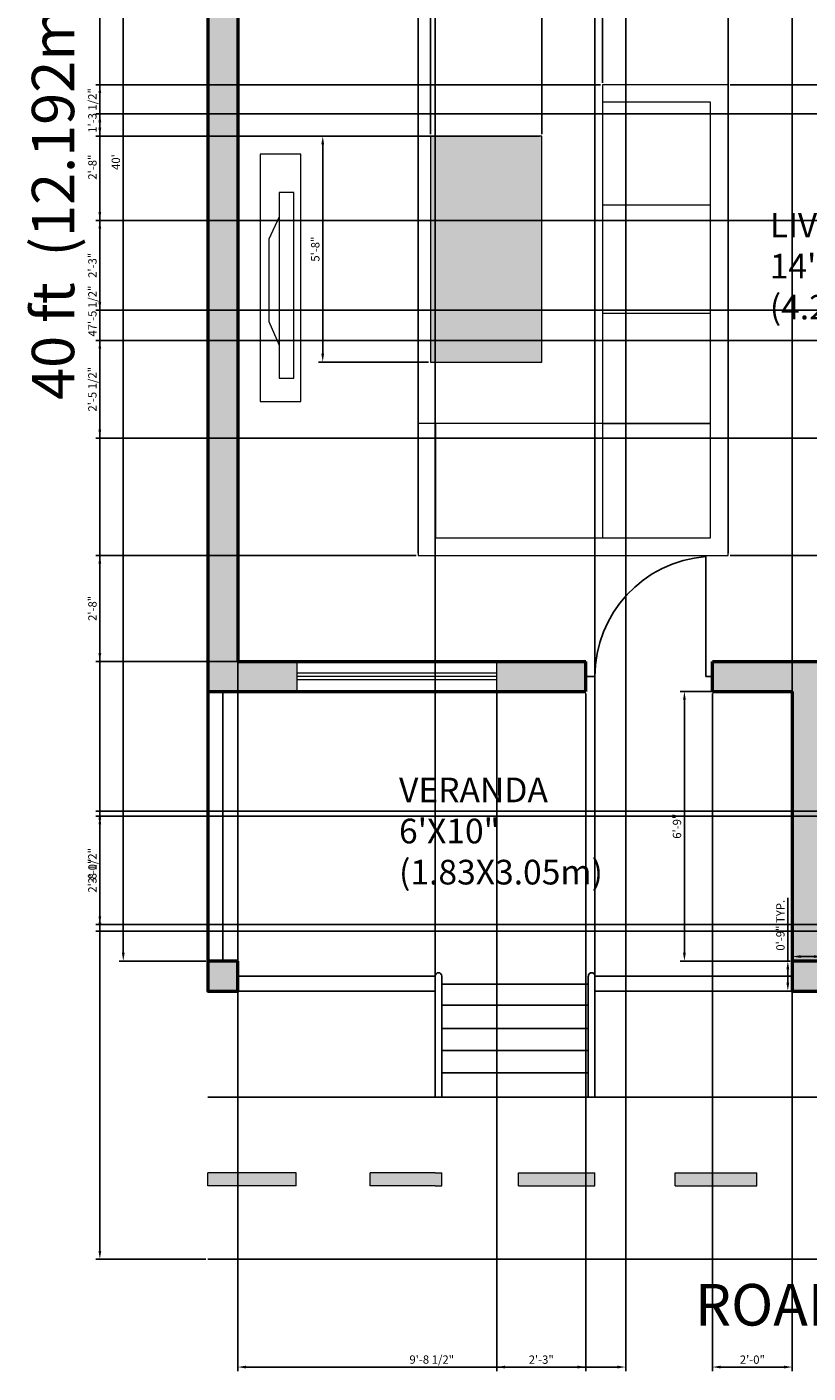
# Model space of a CAD drawing. Units: inches. Extents: x 655 to 1311, y 444 to 1096.
# Tile 1 of 4: x 655 to 890, y 444 to 848. Entities that reach past the tile are written whole.
import ezdxf

# ---------------------------------------------------------------- set-up
doc = ezdxf.new("R2010")
doc.units = ezdxf.units.IN
for name, color, linetype, lineweight in [('A-ANNO-DIMS', 7, 'Continuous', 18), ('A-ANNO-TEXT', 7, 'Continuous', 18), ('A-AREA-IDEN', 7, 'Continuous', 18), ('A-COLS', 7, 'Continuous', 50), ('A-COLS-PATT', 7, 'Continuous', 13), ('A-EQPM', 8, 'Continuous', 18), ('A-FLOR', 7, 'Continuous', 25), ('A-FLOR-STRS', 7, 'Continuous', 25), ('A-WALL', 7, 'Continuous', 50), ('A-WALL-PATT', 7, 'Continuous', 13), ('C-ROAD-MARK', 7, 'Continuous', 13), ('C-ROAD-PATT', 7, 'Continuous', 13)]:
    doc.layers.add(name, color=color, linetype=linetype, lineweight=lineweight)
for name, color, linetype, lineweight, true_color in [('A-DOOR', 251, 'Continuous', 25, 0x636466), ('A-FURN', 251, 'Continuous', 18, 0x636466), ('A-FURN-PATT', 241, 'Continuous', 13, 0xf7abae), ('A-GLAZ', 152, 'Continuous', 18, 0x2776bb), ('C-ROAD', 251, 'Continuous', 25, 0x636466)]:
    doc.layers.add(name, color=color, linetype=linetype, lineweight=lineweight, true_color=true_color)
doc.styles.get("Standard").update_dxf_attribs({"font": 'arial.ttf'})
doc.dimstyles.new('ISO-25', dxfattribs={"dimtxt": 2.5, "dimasz": 2.5, "dimexe": 1.25, "dimexo": 0.625, "dimtad": 1, "dimdec": 0, "dimlunit": 3, "dimtxsty": 'Standard', "dimcen": 2.5, "dimadec": 0, "dimazin": 0, "dimtfac": 1, "dimtdec": 0, "dimtmove": 0, "dimatfit": 3, "dimfxl": 1, "dimarcsym": 0})

# ---------------------------------------------------------------- blocks, each defined once
blk = doc.blocks.new('*D2')
at = {"layer": 'A-ANNO-DIMS', "color": 0, "lineweight": -2, "transparency": 16777216}
for p, q in [((708.71, 1047.75), (682.71, 1047.75)), ((683.96, 570.25), (683.96, 1045.25)), ((708.71, 567.75), (682.71, 567.75))]:
    blk.add_line(p, q, dxfattribs=at)
at = {"layer": 'A-ANNO-DIMS', "color": 0, "transparency": 16777216}
for points in [[(683.55, 1045.25), (684.38, 1045.25), (683.96, 1047.75)], [(683.55, 570.25), (684.38, 570.25), (683.96, 567.75)]]:
    blk.add_solid(points, dxfattribs=at)
at = {"layer": 'Defpoints', "color": 0, "transparency": 16777216}
for p in [(683.96, 1047.75), (709.33, 1047.75), (709.33, 567.75)]:
    blk.add_point(p, dxfattribs=at)
at = {"layer": 'A-ANNO-DIMS', "color": 0, "transparency": 16777216, "insert": (682.06, 807.75), "char_height": 2.5, "attachment_point": 5, "rotation": 90}
blk.add_mtext("40'", dxfattribs=at)
blk = doc.blocks.new('DOOR-SWING-36IN')
for p, q in [((0, 0), (0, 36)), ((-36, 0), (-33.26, 0)), ((0, 0), (2, 0))]:
    blk.add_line(p, q)
blk.add_arc((2.86, 0), 36.11, 94.5377, 180)
blk = doc.blocks.new('WIN-60IN')
for p, q in [((60, 9), (0, 9)), ((0, 9), (0, 0)), ((60, 0), (60, 9)), ((60, 5.5), (0, 5.5)), ((60, 4.5), (0, 4.5)), ((60, 3.5), (0, 3.5)), ((0, 0), (60, 0))]:
    blk.add_line(p, q)
blk = doc.blocks.new('POST-VERANDA-9IN')
blk.add_line((9, 9), (0, 9))
blk.add_lwpolyline([(0, 9), (0, 0), (9, 0), (9, 9)])
blk = doc.blocks.new('*D16')
at = {"layer": 'A-ANNO-DIMS', "color": 0, "lineweight": -2, "transparency": 16777216}
for p, q in [((884.83, 568.38), (884.83, 570.35)), ((893.83, 568.38), (893.83, 570.35)), ((887.33, 569.1), (891.33, 569.1)), ((893.83, 569.1), (941.28, 569.1))]:
    blk.add_line(p, q, dxfattribs=at)
at = {"layer": 'A-ANNO-DIMS', "color": 0, "transparency": 16777216}
for points in [[(887.33, 569.52), (887.33, 568.69), (884.83, 569.1)], [(891.33, 569.52), (891.33, 568.69), (893.83, 569.1)]]:
    blk.add_solid(points, dxfattribs=at)
at = {"layer": 'Defpoints', "color": 0, "transparency": 16777216}
for p in [(884.83, 567.75), (893.83, 569.1), (893.83, 567.75)]:
    blk.add_point(p, dxfattribs=at)
at = {"layer": 'A-ANNO-DIMS', "color": 0, "transparency": 16777216, "insert": (918.81, 571.02), "char_height": 2.5, "attachment_point": 5}
blk.add_mtext('VERANDA POST 0\'-9" TYP.', dxfattribs=at)
blk = doc.blocks.new('*D17')
at = {"layer": 'A-ANNO-DIMS', "color": 0, "lineweight": -2, "transparency": 16777216}
for p, q in [((883.48, 567.75), (883.48, 586.74)), ((884.21, 567.75), (882.23, 567.75)), ((883.48, 561.25), (883.48, 565.25)), ((884.21, 558.75), (882.23, 558.75))]:
    blk.add_line(p, q, dxfattribs=at)
at = {"layer": 'A-ANNO-DIMS', "color": 0, "transparency": 16777216}
for points in [[(883.07, 565.25), (883.9, 565.25), (883.48, 567.75)], [(883.07, 561.25), (883.9, 561.25), (883.48, 558.75)]]:
    blk.add_solid(points, dxfattribs=at)
at = {"layer": 'Defpoints', "color": 0, "transparency": 16777216}
for p in [(883.48, 567.75), (884.83, 567.75), (884.83, 558.75)]:
    blk.add_point(p, dxfattribs=at)
at = {"layer": 'A-ANNO-DIMS', "color": 0, "transparency": 16777216, "insert": (881.58, 578.5), "char_height": 2.5, "attachment_point": 5, "rotation": 90}
blk.add_mtext('0\'-9" TYP.', dxfattribs=at)
blk = doc.blocks.new('*D21')
at = {"layer": 'A-ANNO-DIMS', "color": 0, "lineweight": -2, "transparency": 16777216}
for p, q in [((718.33, 894.13), (718.33, 444.55)), ((834.83, 894.13), (834.83, 444.55)), ((720.83, 445.8), (832.33, 445.8))]:
    blk.add_line(p, q, dxfattribs=at)
at = {"layer": 'A-ANNO-DIMS', "color": 0, "transparency": 16777216}
for points in [[(720.83, 446.22), (720.83, 445.38), (718.33, 445.8)], [(832.33, 446.22), (832.33, 445.38), (834.83, 445.8)]]:
    blk.add_solid(points, dxfattribs=at)
at = {"layer": 'Defpoints', "color": 0, "transparency": 16777216}
for p in [(718.33, 894.75), (834.83, 894.75), (834.83, 445.8)]:
    blk.add_point(p, dxfattribs=at)
at = {"layer": 'A-ANNO-DIMS', "color": 0, "transparency": 16777216, "insert": (776.58, 447.72), "char_height": 2.5, "attachment_point": 5}
blk.add_mtext('9\'-8 1/2"', dxfattribs=at)
blk = doc.blocks.new('*D29')
at = {"layer": 'A-ANNO-DIMS', "color": 0, "lineweight": -2, "transparency": 16777216}
for p, q in [((969.27, 790.23), (675.68, 790.23)), ((676.93, 765.73), (676.93, 787.73)), ((969.27, 763.23), (675.68, 763.23))]:
    blk.add_line(p, q, dxfattribs=at)
at = {"layer": 'A-ANNO-DIMS', "color": 0, "transparency": 16777216}
for points in [[(676.52, 787.73), (677.35, 787.73), (676.93, 790.23)], [(676.52, 765.73), (677.35, 765.73), (676.93, 763.23)]]:
    blk.add_solid(points, dxfattribs=at)
at = {"layer": 'Defpoints', "color": 0, "transparency": 16777216}
for p in [(676.93, 790.23), (969.89, 790.23), (969.89, 763.23)]:
    blk.add_point(p, dxfattribs=at)
at = {"layer": 'A-ANNO-DIMS', "color": 0, "transparency": 16777216, "insert": (675.03, 776.73), "char_height": 2.5, "attachment_point": 5, "rotation": 90}
blk.add_mtext('2\'-3"', dxfattribs=at)
blk = doc.blocks.new('*D30')
at = {"layer": 'A-ANNO-DIMS', "color": 0, "lineweight": -2, "transparency": 16777216}
for p, q in [((969.27, 822.23), (675.68, 822.23)), ((676.93, 792.73), (676.93, 819.73)), ((969.27, 790.23), (675.68, 790.23))]:
    blk.add_line(p, q, dxfattribs=at)
at = {"layer": 'A-ANNO-DIMS', "color": 0, "transparency": 16777216}
for points in [[(676.52, 819.73), (677.35, 819.73), (676.93, 822.23)], [(676.52, 792.73), (677.35, 792.73), (676.93, 790.23)]]:
    blk.add_solid(points, dxfattribs=at)
at = {"layer": 'Defpoints', "color": 0, "transparency": 16777216}
for p in [(676.93, 822.23), (969.89, 822.23), (969.89, 790.23)]:
    blk.add_point(p, dxfattribs=at)
at = {"layer": 'A-ANNO-DIMS', "color": 0, "transparency": 16777216, "insert": (675.03, 806.23), "char_height": 2.5, "attachment_point": 5, "rotation": 90}
blk.add_mtext('2\'-8"', dxfattribs=at)
blk = doc.blocks.new('*D38')
at = {"layer": 'A-ANNO-DIMS', "color": 0, "lineweight": -2, "transparency": 16777216}
for p, q in [((969.27, 754.19), (675.68, 754.19)), ((676.93, 727.35), (676.93, 751.69)), ((969.27, 724.85), (675.68, 724.85))]:
    blk.add_line(p, q, dxfattribs=at)
at = {"layer": 'A-ANNO-DIMS', "color": 0, "transparency": 16777216}
for points in [[(676.52, 751.69), (677.35, 751.69), (676.93, 754.19)], [(676.52, 727.35), (677.35, 727.35), (676.93, 724.85)]]:
    blk.add_solid(points, dxfattribs=at)
at = {"layer": 'Defpoints', "color": 0, "transparency": 16777216}
for p in [(676.93, 754.19), (969.89, 754.19), (969.89, 724.85)]:
    blk.add_point(p, dxfattribs=at)
at = {"layer": 'A-ANNO-DIMS', "color": 0, "transparency": 16777216, "insert": (675.01, 739.52), "char_height": 2.5, "attachment_point": 5, "rotation": 90}
blk.add_mtext('2\'-5 1/2"', dxfattribs=at)
blk = doc.blocks.new('*D39')
at = {"layer": 'A-ANNO-DIMS', "color": 0, "lineweight": -2, "transparency": 16777216}
for p, q in [((902.21, 612.75), (675.68, 612.75)), ((676.93, 579.25), (676.93, 610.25)), ((902.21, 576.75), (675.68, 576.75))]:
    blk.add_line(p, q, dxfattribs=at)
at = {"layer": 'A-ANNO-DIMS', "color": 0, "transparency": 16777216}
for points in [[(676.52, 610.25), (677.35, 610.25), (676.93, 612.75)], [(676.52, 579.25), (677.35, 579.25), (676.93, 576.75)]]:
    blk.add_solid(points, dxfattribs=at)
at = {"layer": 'Defpoints', "color": 0, "transparency": 16777216}
for p in [(676.93, 612.75), (902.83, 612.75), (902.83, 576.75)]:
    blk.add_point(p, dxfattribs=at)
at = {"layer": 'A-ANNO-DIMS', "color": 0, "transparency": 16777216, "insert": (675.03, 594.75), "char_height": 2.5, "attachment_point": 5, "rotation": 90}
blk.add_mtext('3\'-0"', dxfattribs=at)
blk = doc.blocks.new('*D45')
at = {"layer": 'A-ANNO-DIMS', "color": 0, "lineweight": -2, "transparency": 16777216}
for p, q in [((949.58, 611.29), (675.68, 611.29)), ((676.93, 581.21), (676.93, 608.79)), ((949.58, 578.71), (675.68, 578.71))]:
    blk.add_line(p, q, dxfattribs=at)
at = {"layer": 'A-ANNO-DIMS', "color": 0, "transparency": 16777216}
for points in [[(676.52, 608.79), (677.35, 608.79), (676.93, 611.29)], [(676.52, 581.21), (677.35, 581.21), (676.93, 578.71)]]:
    blk.add_solid(points, dxfattribs=at)
at = {"layer": 'Defpoints', "color": 0, "transparency": 16777216}
for p in [(676.93, 611.29), (950.2, 611.29), (950.2, 578.71)]:
    blk.add_point(p, dxfattribs=at)
at = {"layer": 'A-ANNO-DIMS', "color": 0, "transparency": 16777216, "insert": (675.01, 595), "char_height": 2.5, "attachment_point": 5, "rotation": 90}
blk.add_mtext('2\'-8 1/2"', dxfattribs=at)
blk = doc.blocks.new('*D47')
at = {"layer": 'A-ANNO-DIMS', "color": 0, "lineweight": -2, "transparency": 16777216}
for p, q in [((884.21, 648.75), (851.18, 648.75)), ((852.43, 570.25), (852.43, 646.25)), ((884.21, 567.75), (851.18, 567.75))]:
    blk.add_line(p, q, dxfattribs=at)
at = {"layer": 'A-ANNO-DIMS', "color": 0, "transparency": 16777216}
for points in [[(852.02, 646.25), (852.85, 646.25), (852.43, 648.75)], [(852.02, 570.25), (852.85, 570.25), (852.43, 567.75)]]:
    blk.add_solid(points, dxfattribs=at)
at = {"layer": 'Defpoints', "color": 0, "transparency": 16777216}
for p in [(852.43, 648.75), (884.83, 648.75), (884.83, 567.75)]:
    blk.add_point(p, dxfattribs=at)
at = {"layer": 'A-ANNO-DIMS', "color": 0, "transparency": 16777216, "insert": (850.53, 608.25), "char_height": 2.5, "attachment_point": 5, "rotation": 90}
blk.add_mtext('6\'-9"', dxfattribs=at)
blk = doc.blocks.new('*D48')
at = {"layer": 'A-ANNO-DIMS', "color": 0, "lineweight": -2, "transparency": 16777216}
for p, q in [((709.33, 568.38), (709.33, 1081.4)), ((711.83, 1080.15), (882.33, 1080.15)), ((884.83, 568.38), (884.83, 1081.4))]:
    blk.add_line(p, q, dxfattribs=at)
at = {"layer": 'A-ANNO-DIMS', "color": 0, "transparency": 16777216}
for points in [[(711.83, 1080.57), (711.83, 1079.74), (709.33, 1080.15)], [(882.33, 1080.57), (882.33, 1079.74), (884.83, 1080.15)]]:
    blk.add_solid(points, dxfattribs=at)
at = {"layer": 'Defpoints', "color": 0, "transparency": 16777216}
for p in [(884.83, 1080.15), (709.33, 567.75), (884.83, 567.75)]:
    blk.add_point(p, dxfattribs=at)
at = {"layer": 'A-ANNO-DIMS', "color": 0, "transparency": 16777216, "insert": (797.08, 1082.07), "char_height": 2.5, "attachment_point": 5}
blk.add_mtext('14\'-7 1/2"', dxfattribs=at)
blk = doc.blocks.new('*D49')
at = {"layer": 'A-ANNO-DIMS', "color": 0, "lineweight": -2, "transparency": 16777216}
for p, q in [((860.83, 648.13), (860.83, 444.55)), ((884.83, 648.13), (884.83, 444.55)), ((863.33, 445.8), (882.33, 445.8))]:
    blk.add_line(p, q, dxfattribs=at)
at = {"layer": 'A-ANNO-DIMS', "color": 0, "transparency": 16777216}
for points in [[(863.33, 446.22), (863.33, 445.38), (860.83, 445.8)], [(882.33, 446.22), (882.33, 445.38), (884.83, 445.8)]]:
    blk.add_solid(points, dxfattribs=at)
at = {"layer": 'Defpoints', "color": 0, "transparency": 16777216}
for p in [(860.83, 648.75), (884.83, 648.75), (884.83, 445.8)]:
    blk.add_point(p, dxfattribs=at)
at = {"layer": 'A-ANNO-DIMS', "color": 0, "transparency": 16777216, "insert": (872.83, 447.7), "char_height": 2.5, "attachment_point": 5}
blk.add_mtext('2\'-0"', dxfattribs=at)
blk = doc.blocks.new('*D50')
at = {"layer": 'A-ANNO-DIMS', "color": 0, "lineweight": -2, "transparency": 16777216}
for p, q in [((796.08, 648.13), (796.08, 444.55)), ((822.83, 648.13), (822.83, 444.55)), ((798.58, 445.8), (820.33, 445.8))]:
    blk.add_line(p, q, dxfattribs=at)
at = {"layer": 'A-ANNO-DIMS', "color": 0, "transparency": 16777216}
for points in [[(798.58, 446.22), (798.58, 445.38), (796.08, 445.8)], [(820.33, 446.22), (820.33, 445.38), (822.83, 445.8)]]:
    blk.add_solid(points, dxfattribs=at)
at = {"layer": 'Defpoints', "color": 0, "transparency": 16777216}
for p in [(796.08, 648.75), (822.83, 648.75), (822.83, 445.8)]:
    blk.add_point(p, dxfattribs=at)
at = {"layer": 'A-ANNO-DIMS', "color": 0, "transparency": 16777216, "insert": (809.46, 447.7), "char_height": 2.5, "attachment_point": 5}
blk.add_mtext('2\'-3"', dxfattribs=at)
blk = doc.blocks.new('*D51')
at = {"layer": 'A-ANNO-DIMS', "color": 0, "lineweight": -2, "transparency": 16777216}
for p, q in [((718.33, 559.38), (718.33, 1081.4)), ((720.83, 1080.15), (775.08, 1080.15)), ((777.58, 559.38), (777.58, 1081.4))]:
    blk.add_line(p, q, dxfattribs=at)
at = {"layer": 'A-ANNO-DIMS', "color": 0, "transparency": 16777216}
for points in [[(720.83, 1080.57), (720.83, 1079.74), (718.33, 1080.15)], [(775.08, 1080.57), (775.08, 1079.74), (777.58, 1080.15)]]:
    blk.add_solid(points, dxfattribs=at)
at = {"layer": 'Defpoints', "color": 0, "transparency": 16777216}
for p in [(777.58, 1080.15), (718.33, 558.75), (777.58, 558.75)]:
    blk.add_point(p, dxfattribs=at)
at = {"layer": 'A-ANNO-DIMS', "color": 0, "transparency": 16777216, "insert": (747.96, 1082.07), "char_height": 2.5, "attachment_point": 5}
blk.add_mtext('4\'-11 1/2"', dxfattribs=at)
blk = doc.blocks.new('*D53')
at = {"layer": 'A-ANNO-DIMS', "color": 0, "lineweight": -2, "transparency": 16777216}
for p, q in [((777.58, 527.53), (777.58, 1081.4)), ((780.08, 1080.15), (823.08, 1080.15)), ((825.58, 527.53), (825.58, 1081.4))]:
    blk.add_line(p, q, dxfattribs=at)
at = {"layer": 'A-ANNO-DIMS', "color": 0, "transparency": 16777216}
for points in [[(780.08, 1080.57), (780.08, 1079.74), (777.58, 1080.15)], [(823.08, 1080.57), (823.08, 1079.74), (825.58, 1080.15)]]:
    blk.add_solid(points, dxfattribs=at)
at = {"layer": 'Defpoints', "color": 0, "transparency": 16777216}
for p in [(825.58, 1080.15), (777.58, 526.9), (825.58, 526.9)]:
    blk.add_point(p, dxfattribs=at)
at = {"layer": 'A-ANNO-DIMS', "color": 0, "transparency": 16777216, "insert": (801.58, 1082.05), "char_height": 2.5, "attachment_point": 5}
blk.add_mtext('4\'-0"', dxfattribs=at)
blk = doc.blocks.new('*D54')
at = {"layer": 'A-ANNO-DIMS', "color": 0, "lineweight": -2, "transparency": 16777216}
for p, q in [((708.71, 1047.75), (675.68, 1047.75)), ((676.93, 480.7), (676.93, 1045.25)), ((708.71, 478.2), (675.68, 478.2))]:
    blk.add_line(p, q, dxfattribs=at)
at = {"layer": 'A-ANNO-DIMS', "color": 0, "transparency": 16777216}
for points in [[(676.52, 1045.25), (677.35, 1045.25), (676.93, 1047.75)], [(676.52, 480.7), (677.35, 480.7), (676.93, 478.2)]]:
    blk.add_solid(points, dxfattribs=at)
at = {"layer": 'Defpoints', "color": 0, "transparency": 16777216}
for p in [(676.93, 1047.75), (709.33, 1047.75), (709.33, 478.2)]:
    blk.add_point(p, dxfattribs=at)
at = {"layer": 'A-ANNO-DIMS', "color": 0, "transparency": 16777216, "insert": (675.01, 762.98), "char_height": 2.5, "attachment_point": 5, "rotation": 90}
blk.add_mtext('47\'-5 1/2"', dxfattribs=at)
blk = doc.blocks.new('*D55')
at = {"layer": 'A-ANNO-DIMS', "color": 0, "lineweight": -2, "transparency": 16777216}
for p, q in [((772.49, 690.25), (772.49, 1081.4)), ((774.99, 1080.15), (863.04, 1080.15)), ((865.54, 690.25), (865.54, 1081.4))]:
    blk.add_line(p, q, dxfattribs=at)
at = {"layer": 'A-ANNO-DIMS', "color": 0, "transparency": 16777216}
for points in [[(774.99, 1080.57), (774.99, 1079.74), (772.49, 1080.15)], [(863.04, 1080.57), (863.04, 1079.74), (865.54, 1080.15)]]:
    blk.add_solid(points, dxfattribs=at)
at = {"layer": 'Defpoints', "color": 0, "transparency": 16777216}
for p in [(865.54, 1080.15), (772.49, 689.62), (865.54, 689.62)]:
    blk.add_point(p, dxfattribs=at)
at = {"layer": 'A-ANNO-DIMS', "color": 0, "transparency": 16777216, "insert": (819.01, 1082.05), "char_height": 2.5, "attachment_point": 5}
blk.add_mtext('7\'-9"', dxfattribs=at)
blk = doc.blocks.new('*D56')
at = {"layer": 'A-ANNO-DIMS', "color": 0, "lineweight": -2, "transparency": 16777216}
for p, q in [((866.17, 830.95), (899.19, 830.95)), ((897.94, 828.45), (897.94, 692.12)), ((866.17, 689.62), (899.19, 689.62))]:
    blk.add_line(p, q, dxfattribs=at)
at = {"layer": 'A-ANNO-DIMS', "color": 0, "transparency": 16777216}
for points in [[(897.53, 828.45), (898.36, 828.45), (897.94, 830.95)], [(897.53, 692.12), (898.36, 692.12), (897.94, 689.62)]]:
    blk.add_solid(points, dxfattribs=at)
at = {"layer": 'Defpoints', "color": 0, "transparency": 16777216}
for p in [(865.54, 830.95), (865.54, 689.62), (897.94, 689.62)]:
    blk.add_point(p, dxfattribs=at)
at = {"layer": 'A-ANNO-DIMS', "color": 0, "transparency": 16777216, "insert": (896.03, 760.29), "char_height": 2.5, "attachment_point": 5, "rotation": 90}
blk.add_mtext('11\'-9 1/2"', dxfattribs=at)
blk = doc.blocks.new('*D57')
at = {"layer": 'A-ANNO-DIMS', "color": 0, "lineweight": -2, "transparency": 16777216}
for p, q in [((776.25, 816.16), (776.25, 1081.4)), ((778.75, 1080.15), (807.08, 1080.15)), ((809.58, 816.16), (809.58, 1081.4))]:
    blk.add_line(p, q, dxfattribs=at)
at = {"layer": 'A-ANNO-DIMS', "color": 0, "transparency": 16777216}
for points in [[(778.75, 1080.57), (778.75, 1079.74), (776.25, 1080.15)], [(807.08, 1080.57), (807.08, 1079.74), (809.58, 1080.15)]]:
    blk.add_solid(points, dxfattribs=at)
at = {"layer": 'Defpoints', "color": 0, "transparency": 16777216}
for p in [(809.58, 1080.15), (776.25, 815.54), (809.58, 815.54)]:
    blk.add_point(p, dxfattribs=at)
at = {"layer": 'A-ANNO-DIMS', "color": 0, "transparency": 16777216, "insert": (792.91, 1082.07), "char_height": 2.5, "attachment_point": 5}
blk.add_mtext('2\'-9 1/2"', dxfattribs=at)
blk = doc.blocks.new('*D58')
at = {"layer": 'A-ANNO-DIMS', "color": 0, "lineweight": -2, "transparency": 16777216}
for p, q in [((775.62, 815.54), (742.6, 815.54)), ((743.85, 750.17), (743.85, 813.04)), ((775.62, 747.67), (742.6, 747.67))]:
    blk.add_line(p, q, dxfattribs=at)
at = {"layer": 'A-ANNO-DIMS', "color": 0, "transparency": 16777216}
for points in [[(743.43, 813.04), (744.26, 813.04), (743.85, 815.54)], [(743.43, 750.17), (744.26, 750.17), (743.85, 747.67)]]:
    blk.add_solid(points, dxfattribs=at)
at = {"layer": 'Defpoints', "color": 0, "transparency": 16777216}
for p in [(743.85, 815.54), (776.25, 815.54), (776.25, 747.67)]:
    blk.add_point(p, dxfattribs=at)
at = {"layer": 'A-ANNO-DIMS', "color": 0, "transparency": 16777216, "insert": (741.94, 781.6), "char_height": 2.5, "attachment_point": 5, "rotation": 90}
blk.add_mtext('5\'-8"', dxfattribs=at)
blk = doc.blocks.new('*D59')
at = {"layer": 'A-ANNO-DIMS', "color": 0, "lineweight": -2, "transparency": 16777216}
for p, q in [((718.33, 658.38), (718.33, 1081.4)), ((720.83, 1080.15), (769.99, 1080.15)), ((772.49, 690.25), (772.49, 1081.4))]:
    blk.add_line(p, q, dxfattribs=at)
at = {"layer": 'A-ANNO-DIMS', "color": 0, "transparency": 16777216}
for points in [[(720.83, 1080.57), (720.83, 1079.74), (718.33, 1080.15)], [(769.99, 1080.57), (769.99, 1079.74), (772.49, 1080.15)]]:
    blk.add_solid(points, dxfattribs=at)
at = {"layer": 'Defpoints', "color": 0, "transparency": 16777216}
for p in [(772.49, 1080.15), (772.49, 689.62), (718.33, 657.75)]:
    blk.add_point(p, dxfattribs=at)
at = {"layer": 'A-ANNO-DIMS', "color": 0, "transparency": 16777216, "insert": (745.41, 1082.05), "char_height": 2.5, "attachment_point": 5}
blk.add_mtext('4\'-6"', dxfattribs=at)
blk = doc.blocks.new('*D60')
at = {"layer": 'A-ANNO-DIMS', "color": 0, "lineweight": -2, "transparency": 16777216}
for p, q in [((771.86, 689.62), (675.68, 689.62)), ((676.93, 660.25), (676.93, 687.12)), ((822.21, 657.75), (675.68, 657.75))]:
    blk.add_line(p, q, dxfattribs=at)
at = {"layer": 'A-ANNO-DIMS', "color": 0, "transparency": 16777216}
for points in [[(676.52, 687.12), (677.35, 687.12), (676.93, 689.62)], [(676.52, 660.25), (677.35, 660.25), (676.93, 657.75)]]:
    blk.add_solid(points, dxfattribs=at)
at = {"layer": 'Defpoints', "color": 0, "transparency": 16777216}
for p in [(676.93, 689.62), (772.49, 689.62), (822.83, 657.75)]:
    blk.add_point(p, dxfattribs=at)
at = {"layer": 'A-ANNO-DIMS', "color": 0, "transparency": 16777216, "insert": (675.03, 673.69), "char_height": 2.5, "attachment_point": 5, "rotation": 90}
blk.add_mtext('2\'-8"', dxfattribs=at)
blk = doc.blocks.new('*D61')
at = {"layer": 'A-ANNO-DIMS', "color": 0, "lineweight": -2, "transparency": 16777216}
for p, q in [((809.58, 816.16), (809.58, 1081.4)), ((812.08, 1080.15), (825.34, 1080.15)), ((827.84, 831.58), (827.84, 1081.4))]:
    blk.add_line(p, q, dxfattribs=at)
at = {"layer": 'A-ANNO-DIMS', "color": 0, "transparency": 16777216}
for points in [[(812.08, 1080.57), (812.08, 1079.74), (809.58, 1080.15)], [(825.34, 1080.57), (825.34, 1079.74), (827.84, 1080.15)]]:
    blk.add_solid(points, dxfattribs=at)
at = {"layer": 'Defpoints', "color": 0, "transparency": 16777216}
for p in [(827.84, 1080.15), (827.84, 830.95), (809.58, 815.54)]:
    blk.add_point(p, dxfattribs=at)
at = {"layer": 'A-ANNO-DIMS', "color": 0, "transparency": 16777216, "insert": (818.71, 1082.07), "char_height": 2.5, "attachment_point": 5}
blk.add_mtext('1\'-6 1/2"', dxfattribs=at)
blk = doc.blocks.new('*D62')
at = {"layer": 'A-ANNO-DIMS', "color": 0, "lineweight": -2, "transparency": 16777216}
for p, q in [((827.21, 830.95), (675.68, 830.95)), ((676.93, 818.04), (676.93, 828.45)), ((808.95, 815.54), (675.68, 815.54))]:
    blk.add_line(p, q, dxfattribs=at)
at = {"layer": 'A-ANNO-DIMS', "color": 0, "transparency": 16777216}
for points in [[(676.52, 828.45), (677.35, 828.45), (676.93, 830.95)], [(676.52, 818.04), (677.35, 818.04), (676.93, 815.54)]]:
    blk.add_solid(points, dxfattribs=at)
at = {"layer": 'Defpoints', "color": 0, "transparency": 16777216}
for p in [(676.93, 830.95), (827.84, 830.95), (809.58, 815.54)]:
    blk.add_point(p, dxfattribs=at)
at = {"layer": 'A-ANNO-DIMS', "color": 0, "transparency": 16777216, "insert": (675.01, 823.25), "char_height": 2.5, "attachment_point": 5, "rotation": 90}
blk.add_mtext('1\'-3 1/2"', dxfattribs=at)

msp = doc.modelspace()

# ---------------------------------------------------------------- hatches: boundary and pattern name
at = {"layer": 'A-COLS-PATT'}
h = msp.add_hatch(color=256, dxfattribs=at)
h.dxf.hatch_style = 1
h.paths.add_polyline_path([(718.33, 558.75), (718.33, 567.75), (709.33, 567.75), (709.33, 558.75)])
h.paths.add_polyline_path([(893.83, 567.75), (884.83, 567.75), (884.83, 558.75), (893.83, 558.75)])
h.paths.add_polyline_path([(875.1, 756.19), (944.53, 756.19), (944.53, 796.18), (875.1, 796.18)], flags=9)
h.paths.add_polyline_path([(997.04, 810.04), (1045.86, 810.04), (1045.86, 839.51), (997.04, 839.51)], flags=9)
h.paths.add_polyline_path([(949.57, 925.87), (1005.17, 925.87), (1005.17, 959.21), (949.57, 959.21)], flags=9)
h.paths.add_polyline_path([(762.7, 920.37), (822.54, 920.37), (822.54, 956.25), (762.7, 956.25)], flags=9)
at = {"layer": 'A-FURN-PATT'}
h = msp.add_hatch(color=256, dxfattribs=at)
h.dxf.hatch_style = 1
h.paths.add_polyline_path([(809.58, 815.54), (776.25, 815.54), (776.25, 747.67), (809.58, 747.67)])
at = {"layer": 'A-WALL-PATT'}
h = msp.add_hatch(color=256, dxfattribs=at)
h.dxf.hatch_style = 1
h.paths.add_polyline_path([(969.89, 885.75), (1060.33, 885.75), (1060.33, 847.5), (1069.33, 847.5), (1069.33, 1047.75), (1007.08, 1047.75), (1007.08, 1038.75), (1060.33, 1038.75), (1060.33, 894.75), (943.83, 894.75), (943.83, 885.75), (960.89, 885.75), (960.89, 822.23), (969.89, 822.23)])
h.paths.add_polyline_path([(969.89, 780.75), (969.89, 790.23), (960.89, 790.23), (960.89, 733.85), (893.83, 733.85), (893.83, 695.8), (902.83, 695.71), (902.83, 724.85), (969.89, 724.85), (969.89, 754.19), (1060.33, 754.19), (1060.33, 699.99), (1069.33, 699.99), (1069.33, 823.5), (1060.33, 823.5), (1060.33, 763.19), (969.89, 763.19)])
h.paths.add_polyline_path([(947.08, 1047.75), (821.27, 1047.75), (821.27, 1038.75), (884.83, 1038.75), (884.83, 976.7), (884.83, 894.75), (872.83, 894.75), (872.83, 885.75), (905.83, 885.75), (905.83, 894.75), (893.83, 894.75), (893.83, 1038.75), (921.42, 1038.75), (947.08, 1038.75)])
h.paths.add_polyline_path([(761.27, 1047.75), (709.33, 1047.75), (709.33, 648.75), (736.08, 648.75), (736.08, 657.75), (718.33, 657.75), (718.33, 885.75), (834.83, 885.75), (834.83, 894.75), (718.33, 894.75), (718.33, 1038.75), (761.27, 1038.75)])
h.paths.add_polyline_path([(822.83, 657.75), (796.08, 657.75), (796.08, 648.75), (822.83, 648.75)], flags=17)
h.paths.add_polyline_path([(893.83, 657.75), (860.83, 657.75), (860.83, 648.75), (884.83, 648.75), (884.83, 567.75), (893.83, 567.75)])
h.paths.add_polyline_path([(902.83, 657.75), (893.83, 657.75), (893.83, 567.75), (1069.33, 567.75), (1069.33, 639.99), (1060.33, 639.99), (1060.33, 576.75), (902.83, 576.75)])
at = {"layer": 'C-ROAD-PATT'}
h = msp.add_hatch(color=256, dxfattribs=at)
h.dxf.hatch_style = 1
h.paths.add_polyline_path([(735.91, 504.18), (709.33, 504.18), (709.33, 500.25), (735.91, 500.25)])
h.paths.add_polyline_path([(779.58, 504.18), (777.58, 504.18), (758.08, 504.18), (758.08, 500.25), (777.58, 500.25), (779.58, 500.25)])
h.paths.add_polyline_path([(825.58, 504.18), (802.58, 504.18), (802.58, 500.25), (825.58, 500.25)])
h.paths.add_polyline_path([(874.18, 504.18), (849.64, 504.18), (849.64, 500.25), (874.18, 500.25)])
h.paths.add_polyline_path([(969.96, 504.18), (947.46, 504.18), (947.46, 500.25), (969.96, 500.25)])
h.paths.add_polyline_path([(920.36, 504.18), (898.19, 504.18), (898.19, 500.25), (920.36, 500.25)])
h.paths.add_polyline_path([(1020.63, 504.18), (997.93, 504.18), (997.93, 500.25), (1020.63, 500.25)])
h.paths.add_polyline_path([(1069.33, 504.18), (1045.17, 504.18), (1045.17, 500.25), (1069.33, 500.25)])

# ---------------------------------------------------------------- linework, layer by layer
at = {"layer": 'A-EQPM'}
for p, q in [((730.79, 791.32), (727.64, 784.58)), ((727.64, 784.58), (727.64, 759.91)), ((727.64, 759.91), (730.79, 752.8))]:
    msp.add_line(p, q, dxfattribs=at)
msp.add_lwpolyline([(730.79, 742.87), (735.15, 742.87), (735.15, 798.59), (730.79, 798.59)], close=True, dxfattribs=at)
at = {"layer": 'A-FLOR'}
for p, q in [((713.83, 567.75), (713.83, 648.75)), ((718.33, 563.25), (777.59, 563.25)), ((825.58, 563.25), (884.83, 563.25)), ((718.33, 558.75), (777.58, 558.75)), ((825.58, 558.75), (884.83, 558.75))]:
    msp.add_line(p, q, dxfattribs=at)
at = {"layer": 'A-FLOR-STRS'}
for p, q in [((777.58, 563.25), (777.58, 526.9)), ((779.58, 563.25), (779.58, 526.9)), ((779.58, 563.25), (779.58, 563.25)), ((823.58, 563.25), (823.59, 563.25)), ((823.58, 563.25), (823.58, 526.9)), ((825.58, 563.25), (825.58, 526.9)), ((779.58, 560.78), (823.58, 560.78)), ((779.58, 554.54), (823.58, 554.54)), ((779.58, 547.51), (823.58, 547.51)), ((779.58, 540.85), (823.58, 540.85)), ((779.58, 534.16), (823.58, 534.16))]:
    msp.add_line(p, q, dxfattribs=at)
for centre in [(778.58, 563.25), (824.59, 563.25)]:
    msp.add_arc(centre, 0.995, 0, 180, dxfattribs=at)
at = {"layer": 'A-FURN'}
for p, q in [((827.84, 830.95), (827.84, 694.86)), ((865.54, 830.95), (827.84, 830.95)), ((865.54, 689.62), (865.54, 830.95)), ((860.3, 825.71), (827.84, 825.71)), ((860.3, 729.18), (860.3, 825.71)), ((860.3, 794.83), (827.84, 794.83)), ((860.3, 762.31), (827.84, 762.31)), ((860.3, 729.18), (772.49, 729.18)), ((772.49, 729.18), (772.49, 689.62)), ((777.73, 729.18), (777.73, 694.86)), ((827.84, 729.18), (860.3, 729.18)), ((860.3, 694.86), (860.3, 729.18)), ((777.73, 694.86), (860.3, 694.86)), ((772.49, 689.62), (865.54, 689.62))]:
    msp.add_line(p, q, dxfattribs=at)
for points in [[(776.25, 747.67), (809.58, 747.67), (809.58, 815.54), (776.25, 815.54)], [(725.04, 735.81), (737.32, 735.81), (737.32, 810.08), (725.04, 810.08)]]:
    msp.add_lwpolyline(points, close=True, dxfattribs=at)
at = {"layer": 'A-WALL'}
for p, q in [((718.33, 885.75), (718.33, 657.75)), ((718.33, 657.75), (822.83, 657.75)), ((822.83, 648.75), (822.83, 657.75)), ((860.83, 648.75), (860.83, 657.75)), ((860.83, 657.75), (902.83, 657.75)), ((709.33, 648.75), (822.83, 648.75)), ((860.83, 648.75), (884.83, 648.75)), ((884.83, 648.75), (884.83, 567.75))]:
    msp.add_line(p, q, dxfattribs=at)
msp.add_lwpolyline([(893.83, 567.75), (1069.33, 567.75), (1069.33, 1047.75), (709.33, 1047.75), (709.33, 567.75)], dxfattribs=at)
at = {"layer": 'C-ROAD'}
for p, q in [((777.58, 526.9), (709.33, 526.9)), ((779.58, 526.9), (777.58, 526.9)), ((779.58, 526.9), (825.58, 526.9)), ((825.58, 526.9), (1069.33, 526.9)), ((777.58, 478.2), (709.33, 478.2)), ((777.58, 478.2), (779.58, 478.2)), ((779.58, 478.2), (825.58, 478.2)), ((825.58, 478.2), (1069.33, 478.2))]:
    msp.add_line(p, q, dxfattribs=at)
at = {"layer": 'C-ROAD-MARK'}
for p, q in [((709.33, 500.25), (709.33, 504.18)), ((735.91, 504.18), (709.33, 504.18)), ((735.91, 500.25), (735.91, 504.18)), ((777.58, 504.18), (758.08, 504.18)), ((758.08, 500.25), (758.08, 504.18)), ((777.58, 504.18), (779.58, 504.18)), ((779.58, 500.25), (779.58, 504.18)), ((802.58, 504.18), (825.58, 504.18)), ((802.58, 500.25), (802.58, 504.18)), ((825.58, 500.25), (825.58, 504.18)), ((849.64, 504.18), (874.18, 504.18)), ((849.64, 500.25), (849.64, 504.18)), ((874.18, 500.25), (874.18, 504.18)), ((735.91, 500.25), (709.33, 500.25)), ((777.58, 500.25), (758.08, 500.25)), ((777.58, 500.25), (779.58, 500.25)), ((802.58, 500.25), (825.58, 500.25)), ((849.64, 500.25), (874.18, 500.25))]:
    msp.add_line(p, q, dxfattribs=at)

# ---------------------------------------------------------------- block references
at = {"layer": 'A-COLS'}
for p in [(709.33, 558.75), (884.83, 558.75)]:
    msp.add_blockref('POST-VERANDA-9IN', p, dxfattribs=at)
at = {"layer": 'A-DOOR'}
msp.add_blockref('DOOR-SWING-36IN', (858.83, 653.25), dxfattribs=at)
at = {"layer": 'A-GLAZ'}
msp.add_blockref('WIN-60IN', (736.08, 648.75), dxfattribs=at)

# ---------------------------------------------------------------- texts
at = {"layer": 'A-ANNO-DIMS', "insert": (656.52, 736.3), "char_height": 12.7117, "attachment_point": 1, "rotation": 90}
msp.add_mtext_dynamic_manual_height_columns('40 ft  (12.192m)', width=400.2868, gutter_width=63.56, heights=[0], dxfattribs=at)
at = {"layer": 'A-ANNO-TEXT', "insert": (855.63, 470.76), "char_height": 12.499, "attachment_point": 1}
msp.add_mtext_dynamic_manual_height_columns('ROAD', width=237.3876, gutter_width=58.61, heights=[0], dxfattribs=at)
at = {"layer": 'A-AREA-IDEN', "attachment_point": 1}
for s, width, gutter_width, insert, char_height in [("LIVING /HALL\\P14'X16'\\P(4.27X4.88m)", 351.6756, 36.92, (878.07, 792.5), 7.3846), ('VERANDA\\P6\'X10"\\P(1.83X3.05m)', 268.5778, 37.02, (766.75, 622.85), 7.4038)]:
    msp.add_mtext_dynamic_manual_height_columns(s, width=width, gutter_width=gutter_width, heights=[0], dxfattribs=dict(at, insert=insert, char_height=char_height))

# ---------------------------------------------------------------- dimensions: what is measured, and where the dimension line sits
at = {"layer": 'A-ANNO-DIMS'}
for base, p1, p2, picture, middle in [((884.83, 1080.15), (709.33, 567.75), (884.83, 567.75), '*D48', (797.08, 1082.07)), ((777.582624, 1080.153006), (718.332624, 558.753006), (777.582624, 558.753006), '*D51', (747.957624, 1082.07063902)), ((772.49, 1080.15), (718.33, 657.75), (772.49, 689.62), '*D59', (745.41, 1082.05)), ((865.5433, 1080.153), (772.4866, 689.6218), (865.5433, 689.6218), '*D55', (819.0149, 1082.0544)), ((809.58, 1080.15), (776.25, 815.54), (809.58, 815.54), '*D57', (792.91, 1082.07)), ((825.58, 1080.15), (777.58, 526.9), (825.58, 526.9), '*D53', (801.58, 1082.05)), ((827.84, 1080.15), (809.58, 815.54), (827.84, 830.95), '*D61', (818.71, 1082.07)), ((834.83, 445.8), (718.33, 894.75), (834.83, 894.75), '*D21', (776.58, 447.72)), ((822.832624, 445.801021), (796.082624, 648.753006), (822.832624, 648.753006), '*D50', (809.457624, 447.70330613)), ((884.83, 445.8), (860.83, 648.75), (884.83, 648.75), '*D49', (872.83, 447.7))]:
    dim = msp.add_linear_dim(base=base, p1=p1, p2=p2, dimstyle='ISO-25', override={"dimdec": 1, "dimlfac": 1, "dimrnd": 0, "dimzin": 1, "dimdsep": 46, "dimlunit": 4, "dimfrac": 2}, dxfattribs=at)
    dim.commit()
    dim.dimension.update_dxf_attribs({"geometry": picture, "text_midpoint": middle})
for base, p1, p2, angle, override, picture, middle in [((676.9326, 1047.753), (709.3326, 478.201), (709.3326, 1047.753), 90, {"dimdec": 1, "dimlfac": 1, "dimrnd": 0, "dimzin": 1, "dimdsep": 46, "dimlunit": 4, "dimfrac": 2}, '*D54', (675.015, 762.977)), ((683.96, 1047.75), (709.33, 567.75), (709.33, 1047.75), 90, {"dimclrd": 0, "dimclre": 0, "dimclrt": 0}, '*D2', (682.06, 807.75)), ((676.93, 830.95), (809.58, 815.54), (827.84, 830.95), 90, {"dimdec": 1, "dimlfac": 1, "dimrnd": 0, "dimzin": 1, "dimdsep": 46, "dimlunit": 4, "dimfrac": 2}, '*D62', (675.01, 823.25)), ((897.94, 689.62), (865.54, 830.95), (865.54, 689.62), 270, {"dimdec": 1, "dimlfac": 1, "dimrnd": 0, "dimzin": 1, "dimdsep": 46, "dimlunit": 4, "dimfrac": 2}, '*D56', (896.03, 760.29)), ((676.93, 822.23), (969.89, 790.23), (969.89, 822.23), 90, {"dimdec": 1, "dimlfac": 1, "dimrnd": 0, "dimzin": 1, "dimdsep": 46, "dimlunit": 4, "dimfrac": 2}, '*D30', (675.03, 806.23)), ((743.85, 815.54), (776.25, 747.67), (776.25, 815.54), 90, {"dimdec": 1, "dimlfac": 1, "dimrnd": 0, "dimzin": 1, "dimdsep": 46, "dimlunit": 4, "dimfrac": 2}, '*D58', (741.94, 781.6)), ((676.93, 790.23), (969.89, 763.23), (969.89, 790.23), 90, {"dimdec": 1, "dimlfac": 1, "dimrnd": 0, "dimzin": 1, "dimdsep": 46, "dimlunit": 4, "dimfrac": 2}, '*D29', (675.03, 776.73)), ((676.93, 754.19), (969.89, 724.85), (969.89, 754.19), 90, {"dimdec": 1, "dimlfac": 1, "dimrnd": 0, "dimzin": 1, "dimdsep": 46, "dimlunit": 4, "dimfrac": 2}, '*D38', (675.01, 739.52)), ((676.93, 689.62), (822.83, 657.75), (772.49, 689.62), 90, {"dimdec": 1, "dimlfac": 1, "dimrnd": 0, "dimzin": 1, "dimdsep": 46, "dimlunit": 4, "dimfrac": 2}, '*D60', (675.03, 673.69)), ((852.43, 648.75), (884.83, 567.75), (884.83, 648.75), 90, {"dimdec": 1, "dimlfac": 1, "dimrnd": 0, "dimzin": 1, "dimdsep": 46, "dimlunit": 4, "dimfrac": 2}, '*D47', (850.53, 608.25)), ((676.93, 611.29), (950.2, 578.71), (950.2, 611.29), 90, {"dimdec": 1, "dimlfac": 1, "dimrnd": 0, "dimzin": 1, "dimdsep": 46, "dimlunit": 4, "dimfrac": 2}, '*D45', (675.01, 595)), ((676.93, 612.75), (902.83, 576.75), (902.83, 612.75), 90, {"dimdec": 1, "dimlfac": 1, "dimrnd": 0, "dimzin": 1, "dimdsep": 46, "dimlunit": 4, "dimfrac": 2}, '*D39', (675.03, 594.75))]:
    dim = msp.add_linear_dim(base=base, p1=p1, p2=p2, angle=angle, dimstyle='ISO-25', override=override, dxfattribs=at)
    dim.commit()
    dim.dimension.update_dxf_attribs({"geometry": picture, "text_midpoint": middle})
dim = msp.add_linear_dim(base=(883.48, 567.75), p1=(884.83, 558.75), p2=(884.83, 567.75), angle=90, text='<> TYP.', dimstyle='ISO-25', override={"dimdec": 1, "dimlfac": 1, "dimrnd": 0, "dimzin": 1, "dimdsep": 46, "dimlunit": 4, "dimfrac": 2}, dxfattribs=at)
dim.commit()
dim.dimension.update_dxf_attribs({"geometry": '*D17', "text_midpoint": (881.58, 578.5)})
dim = msp.add_linear_dim(base=(893.83, 569.1), p1=(884.83, 567.75), p2=(893.83, 567.75), text='VERANDA POST <> TYP.', dimstyle='ISO-25', override={"dimdec": 1, "dimlfac": 1, "dimrnd": 0, "dimzin": 1, "dimdsep": 46, "dimlunit": 4, "dimfrac": 2}, dxfattribs=at)
dim.commit()
dim.dimension.update_dxf_attribs({"geometry": '*D16', "text_midpoint": (918.81, 571.02)})

doc.saveas('drawing.dxf')
